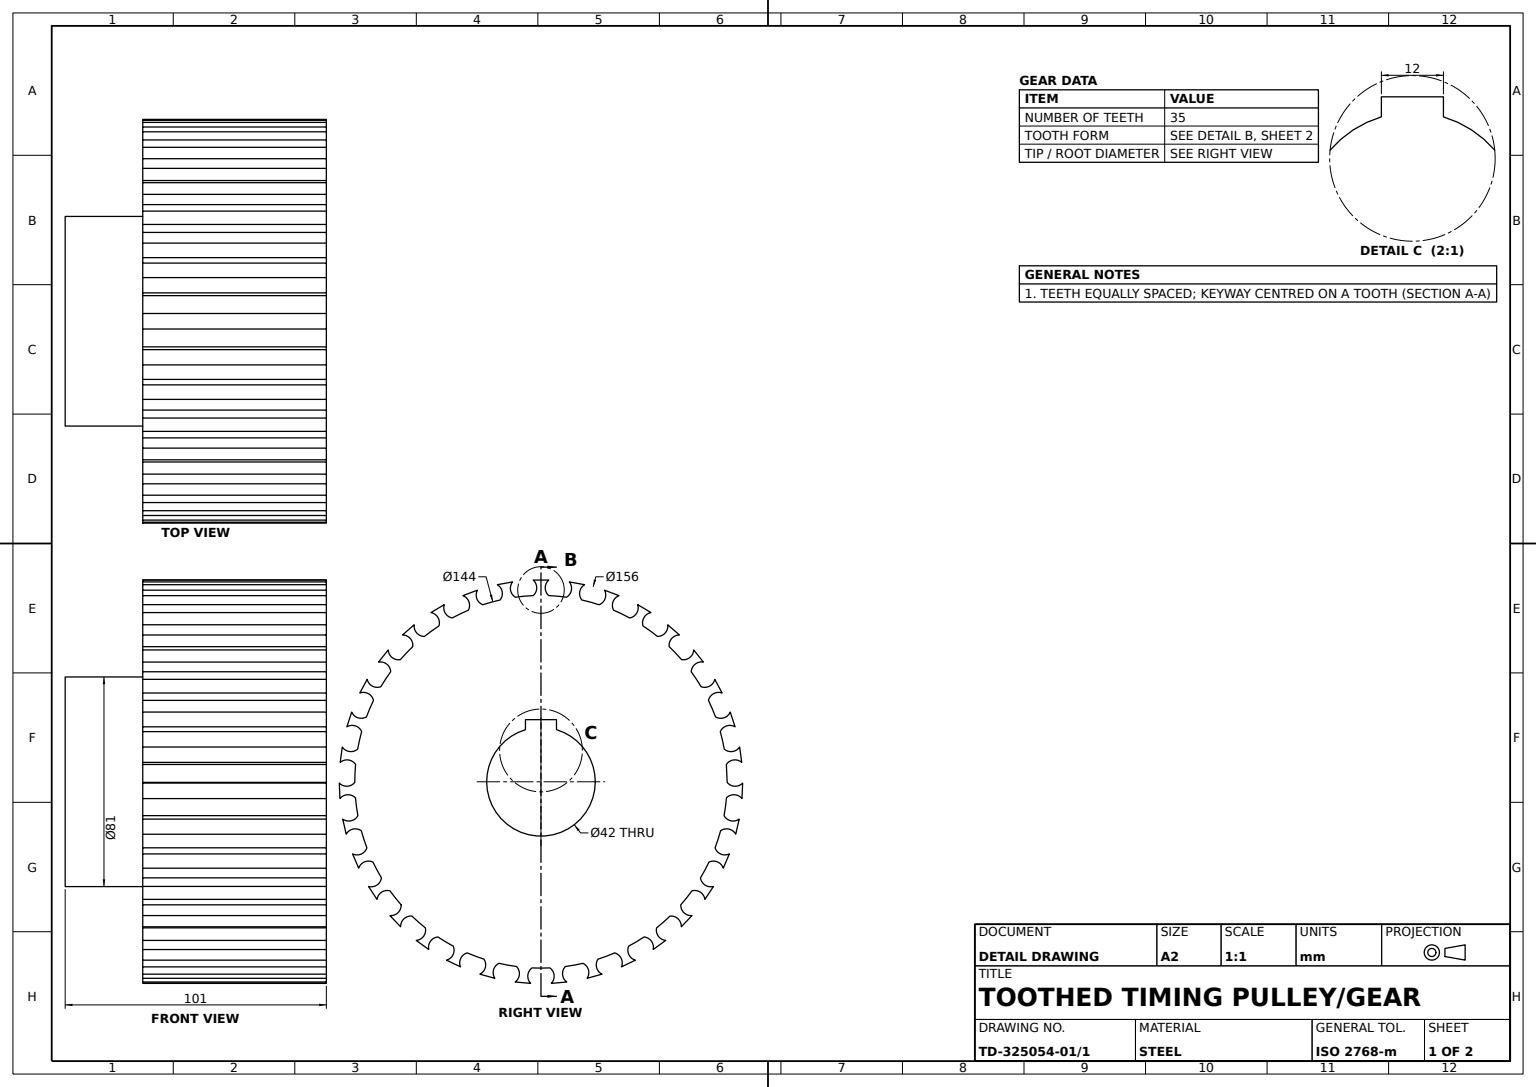
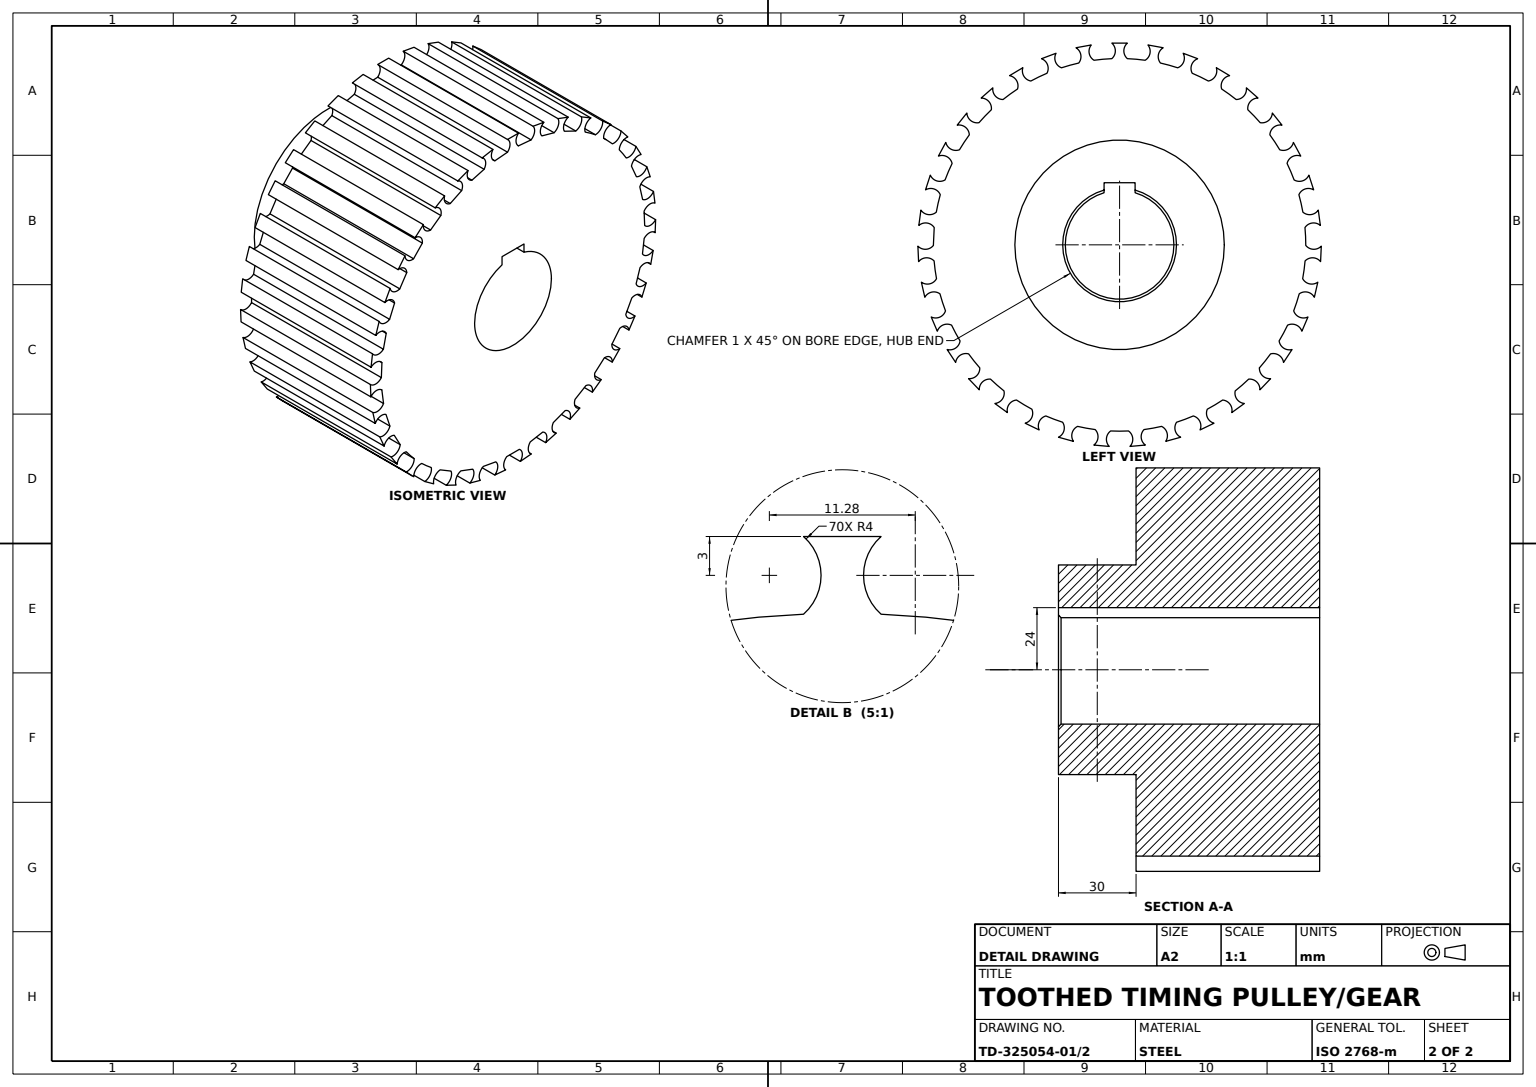
SolidWorks part; units mm, degrees
material "Plain Carbon Steel"
ref_plane "Front Plane" through (0, 0, 0) normal (0, 0, 1) x (1, 0, 0)
ref_plane "Top Plane" through (0, 0, 0) normal (0, 1, 0) x (1, 0, 0)
ref_plane "Right Plane" through (0, 0, 0) normal (1, 0, 0) x (0, 0, -1)
sketch "Gear Tooth Profile Sketch" plane through (0, 0, 0) normal (0, 0, 1) x (1, 0, 0)
  line L0 (0, 0) -> (0, 72) construction
  line L3 (0, 72) -> (0, 83.2045)
  line L4 (-2.9993, 80.7614) -> (-2.9993, 80.6935) construction
  arc A0 (2.9993, 77.9423) -> (-2.9993, 77.9423) centre (0, 0) ccw
  arc A1 (-2.9993, 71.9375) -> (-9.8938, 71.317) centre (0, 0) ccw
  circle A2 centre (0, 0) radius 64.8
  arc A3 (2.9993, 71.9375) -> (2.9993, 77.9423) centre (5.6424, 74.9399) cw
  arc A4 (-2.9993, 71.9375) -> (-2.9993, 77.9423) centre (-5.6424, 74.9399) ccw
  arc A5 (9.8938, 71.317) -> (10.966, 77.2253) centre (7.8293, 74.7431) ccw
  arc A6 (15.7961, 70.2459) -> (16.8683, 76.1542) centre (18.9327, 72.7281) cw
  arc A7 (22.4689, 68.4043) -> (24.5789, 74.0262) centre (21.0494, 72.1439) ccw
  arc A8 (28.0851, 66.2965) -> (30.1951, 71.9184) centre (31.6146, 68.1788) cw
  arc A9 (34.3219, 63.293) -> (37.4018, 68.4478) centre (33.5929, 67.226) ccw
  arc A10 (39.4715, 60.2163) -> (42.5513, 65.3711) centre (43.2803, 61.4381) cw
  arc A11 (45.0717, 56.1475) -> (49.0225, 60.6695) centre (45.0568, 60.1474) ccw
  arc A12 (49.5892, 52.2007) -> (53.54, 56.7227) centre (53.555, 52.7228) cw
  arc A13 (54.3729, 47.1973) -> (59.0677, 50.9412) centre (55.0724, 51.1356) ccw
  arc A14 (58.1131, 42.5073) -> (62.8078, 46.2513) centre (62.1083, 42.3129) cw
  arc A15 (61.9265, 36.7301) -> (67.2144, 39.5756) centre (63.318, 40.4803) ccw
  arc A16 (64.7691, 31.4477) -> (70.0569, 34.2932) centre (68.6655, 30.543) cw
  arc A17 (67.4898, 25.0825) -> (73.2007, 26.938) centre (69.5285, 28.5239) ccw
  arc A18 (69.3435, 19.3774) -> (75.0544, 21.2329) centre (73.0157, 17.7915) cw
  arc A19 (70.8838, 12.6286) -> (76.8343, 13.4347) centre (73.5043, 15.6507) ccw
  arc A20 (71.6891, 6.6842) -> (77.6395, 7.4902) centre (75.0191, 4.4681) cw
  arc A21 (71.9996, -0.2311) -> (77.9984, -0.5005) centre (75.1176, 2.2745) ccw
  arc A22 (71.7305, -6.2238) -> (77.7293, -6.4932) centre (74.6113, -8.9989) cw
  arc A23 (70.8013, -13.0835) -> (76.6556, -14.4196) centre (74.3166, -11.1748) ccw
  arc A24 (69.4665, -18.9317) -> (75.3207, -20.2679) centre (71.8055, -22.1766) cw
  arc A25 (67.3273, -25.5153) -> (72.8489, -27.8753) centre (71.1269, -24.2649) ccw
  arc A26 (64.9697, -31.0312) -> (70.4913, -33.3913) centre (66.6917, -34.6416) cw
  arc A27 (61.6894, -37.127) -> (66.7009, -40.435) centre (65.6512, -36.5752) ccw
  arc A28 (58.3848, -42.1333) -> (63.3962, -45.4414) centre (59.4345, -45.9931) cw
  arc A29 (54.0688, -47.5454) -> (58.409, -51.6951) centre (58.0654, -47.7099) ccw
  arc A30 (49.9233, -51.8812) -> (54.2636, -56.0309) centre (50.2669, -55.8664) cw
  arc A31 (44.7103, -56.4357) -> (48.2399, -61.2937) centre (48.6133, -57.3112) ccw
  arc A32 (39.8573, -59.9616) -> (43.3868, -64.8196) centre (39.4838, -63.9442) cw
  arc A33 (33.9148, -63.5121) -> (36.5202, -68.9222) centre (37.5988, -65.0704) ccw
  arc A34 (28.5102, -66.1148) -> (31.1156, -71.525) centre (27.4316, -69.9667) cw
  arc A35 (22.0293, -68.5471) -> (23.6268, -74.3356) centre (25.3758, -70.7382) ccw
  arc A36 (16.2468, -70.143) -> (17.8443, -75.9314) centre (14.4977, -73.7404) cw
  arc A37 (9.4357, -71.379) -> (9.974, -77.3597) centre (12.3372, -74.1324) ccw
  arc A38 (3.4612, -71.9168) -> (3.9994, -77.8974) centre (1.0979, -75.144) cw
  arc A39 (-3.4612, -71.9168) -> (-3.9994, -77.8974) centre (-1.0979, -75.144) ccw
  arc A40 (-9.4357, -71.379) -> (-9.974, -77.3597) centre (-12.3372, -74.1324) cw
  arc A41 (-16.2468, -70.143) -> (-17.8443, -75.9314) centre (-14.4977, -73.7404) ccw
  arc A42 (-22.0293, -68.5471) -> (-23.6268, -74.3356) centre (-25.3758, -70.7382) cw
  arc A43 (-28.5102, -66.1148) -> (-31.1156, -71.525) centre (-27.4316, -69.9667) ccw
  arc A44 (-33.9148, -63.5121) -> (-36.5202, -68.9222) centre (-37.5988, -65.0704) cw
  arc A45 (-39.8573, -59.9616) -> (-43.3868, -64.8196) centre (-39.4838, -63.9442) ccw
  arc A46 (-44.7103, -56.4357) -> (-48.2399, -61.2937) centre (-48.6133, -57.3112) cw
  arc A47 (-49.9233, -51.8812) -> (-54.2636, -56.0309) centre (-50.2669, -55.8664) ccw
  arc A48 (-54.0688, -47.5454) -> (-58.409, -51.6951) centre (-58.0654, -47.7099) cw
  arc A49 (-58.3848, -42.1333) -> (-63.3962, -45.4414) centre (-59.4345, -45.9931) ccw
  arc A50 (-61.6894, -37.127) -> (-66.7009, -40.435) centre (-65.6512, -36.5752) cw
  arc A51 (-64.9697, -31.0312) -> (-70.4913, -33.3913) centre (-66.6917, -34.6416) ccw
  arc A52 (-67.3273, -25.5153) -> (-72.8489, -27.8753) centre (-71.1269, -24.2649) cw
  arc A53 (-69.4665, -18.9317) -> (-75.3207, -20.2679) centre (-71.8055, -22.1766) ccw
  arc A54 (-70.8013, -13.0835) -> (-76.6556, -14.4196) centre (-74.3166, -11.1748) cw
  arc A55 (-71.7305, -6.2238) -> (-77.7293, -6.4932) centre (-74.6113, -8.9989) ccw
  arc A56 (-71.9996, -0.2311) -> (-77.9984, -0.5005) centre (-75.1176, 2.2745) cw
  arc A57 (-71.6891, 6.6842) -> (-77.6395, 7.4902) centre (-75.0191, 4.4681) ccw
  arc A58 (-70.8838, 12.6286) -> (-76.8343, 13.4347) centre (-73.5043, 15.6507) cw
  arc A59 (-69.3435, 19.3774) -> (-75.0544, 21.2329) centre (-73.0157, 17.7915) ccw
  arc A60 (-67.4898, 25.0825) -> (-73.2007, 26.938) centre (-69.5285, 28.5239) cw
  arc A61 (-64.7691, 31.4477) -> (-70.0569, 34.2932) centre (-68.6655, 30.543) ccw
  arc A62 (-61.9265, 36.7301) -> (-67.2144, 39.5756) centre (-63.318, 40.4803) cw
  arc A63 (-58.1131, 42.5073) -> (-62.8078, 46.2513) centre (-62.1083, 42.3129) ccw
  arc A64 (-54.3729, 47.1973) -> (-59.0677, 50.9412) centre (-55.0724, 51.1356) cw
  arc A65 (-49.5892, 52.2007) -> (-53.54, 56.7227) centre (-53.555, 52.7228) ccw
  arc A66 (-45.0717, 56.1475) -> (-49.0225, 60.6695) centre (-45.0568, 60.1474) cw
  arc A67 (-39.4715, 60.2163) -> (-42.5513, 65.3711) centre (-43.2803, 61.4381) ccw
  arc A68 (-34.3219, 63.293) -> (-37.4018, 68.4478) centre (-33.5929, 67.226) cw
  arc A69 (-28.0851, 66.2965) -> (-30.1951, 71.9184) centre (-31.6146, 68.1788) ccw
  arc A70 (-22.4689, 68.4043) -> (-24.5789, 74.0262) centre (-21.0494, 72.1439) cw
  arc A71 (-15.7961, 70.2459) -> (-16.8683, 76.1542) centre (-18.9327, 72.7281) ccw
  arc A72 (-9.8938, 71.317) -> (-10.966, 77.2253) centre (-7.8293, 74.7431) cw
  arc A73 (16.8683, 76.1542) -> (10.966, 77.2253) centre (0, 0) ccw
  arc A74 (30.1951, 71.9184) -> (24.5789, 74.0262) centre (0, 0) ccw
  arc A75 (42.5513, 65.3711) -> (37.4018, 68.4478) centre (0, 0) ccw
  arc A76 (53.54, 56.7227) -> (49.0225, 60.6695) centre (0, 0) ccw
  arc A77 (62.8078, 46.2513) -> (59.0677, 50.9412) centre (0, 0) ccw
  arc A78 (70.0569, 34.2932) -> (67.2144, 39.5756) centre (0, 0) ccw
  arc A79 (75.0544, 21.2329) -> (73.2007, 26.938) centre (0, 0) ccw
  arc A80 (77.6395, 7.4902) -> (76.8343, 13.4347) centre (0, 0) ccw
  arc A81 (77.7293, -6.4932) -> (77.9984, -0.5005) centre (0, 0) ccw
  arc A82 (75.3207, -20.2679) -> (76.6556, -14.4196) centre (0, 0) ccw
  arc A83 (70.4913, -33.3913) -> (72.8489, -27.8753) centre (0, 0) ccw
  arc A84 (63.3962, -45.4414) -> (66.7009, -40.435) centre (0, 0) ccw
  arc A85 (54.2636, -56.0309) -> (58.409, -51.6951) centre (0, 0) ccw
  arc A86 (43.3868, -64.8196) -> (48.2399, -61.2937) centre (0, 0) ccw
  arc A87 (31.1156, -71.525) -> (36.5202, -68.9222) centre (0, 0) ccw
  arc A88 (17.8443, -75.9314) -> (23.6268, -74.3356) centre (0, 0) ccw
  arc A89 (3.9994, -77.8974) -> (9.974, -77.3597) centre (0, 0) ccw
  arc A90 (-9.974, -77.3597) -> (-3.9994, -77.8974) centre (0, 0) ccw
  arc A91 (-23.6268, -74.3356) -> (-17.8443, -75.9314) centre (0, 0) ccw
  arc A92 (-36.5202, -68.9222) -> (-31.1156, -71.525) centre (0, 0) ccw
  arc A93 (-48.2399, -61.2937) -> (-43.3868, -64.8196) centre (0, 0) ccw
  arc A94 (-58.409, -51.6951) -> (-54.2636, -56.0309) centre (0, 0) ccw
  arc A95 (-66.7009, -40.435) -> (-63.3962, -45.4414) centre (0, 0) ccw
  arc A96 (-72.8489, -27.8753) -> (-70.4913, -33.3913) centre (0, 0) ccw
  arc A97 (-76.6556, -14.4196) -> (-75.3207, -20.2679) centre (0, 0) ccw
  arc A98 (-77.9984, -0.5005) -> (-77.7293, -6.4932) centre (0, 0) ccw
  arc A99 (-76.8343, 13.4347) -> (-77.6395, 7.4902) centre (0, 0) ccw
  arc A100 (-73.2007, 26.938) -> (-75.0544, 21.2329) centre (0, 0) ccw
  arc A101 (-67.2144, 39.5756) -> (-70.0569, 34.2932) centre (0, 0) ccw
  arc A102 (-59.0677, 50.9412) -> (-62.8078, 46.2513) centre (0, 0) ccw
  arc A103 (-49.0225, 60.6695) -> (-53.54, 56.7227) centre (0, 0) ccw
  arc A104 (-37.4018, 68.4478) -> (-42.5513, 65.3711) centre (0, 0) ccw
  arc A105 (-24.5789, 74.0262) -> (-30.1951, 71.9184) centre (0, 0) ccw
  arc A106 (-10.966, 77.2253) -> (-16.8683, 76.1542) centre (0, 0) ccw
  arc A107 (9.8938, 71.317) -> (2.9993, 71.9375) centre (0, 0) ccw
  arc A108 (22.4689, 68.4043) -> (15.7961, 70.2459) centre (0, 0) ccw
  arc A109 (34.3219, 63.293) -> (28.0851, 66.2965) centre (0, 0) ccw
  arc A110 (45.0717, 56.1475) -> (39.4715, 60.2163) centre (0, 0) ccw
  arc A111 (54.3729, 47.1973) -> (49.5892, 52.2007) centre (0, 0) ccw
  arc A112 (61.9265, 36.7301) -> (58.1131, 42.5073) centre (0, 0) ccw
  arc A113 (67.4898, 25.0825) -> (64.7691, 31.4477) centre (0, 0) ccw
  arc A114 (70.8838, 12.6286) -> (69.3435, 19.3774) centre (0, 0) ccw
  arc A115 (71.9996, -0.2311) -> (71.6891, 6.6842) centre (0, 0) ccw
  arc A116 (70.8013, -13.0835) -> (71.7305, -6.2238) centre (0, 0) ccw
  arc A117 (67.3273, -25.5153) -> (69.4665, -18.9317) centre (0, 0) ccw
  arc A118 (61.6894, -37.127) -> (64.9697, -31.0312) centre (0, 0) ccw
  arc A119 (54.0688, -47.5454) -> (58.3848, -42.1333) centre (0, 0) ccw
  arc A120 (44.7103, -56.4357) -> (49.9233, -51.8812) centre (0, 0) ccw
  arc A121 (33.9148, -63.5121) -> (39.8573, -59.9616) centre (0, 0) ccw
  arc A122 (22.0293, -68.5471) -> (28.5102, -66.1148) centre (0, 0) ccw
  arc A123 (9.4357, -71.379) -> (16.2468, -70.143) centre (0, 0) ccw
  arc A124 (-3.4612, -71.9168) -> (3.4612, -71.9168) centre (0, 0) ccw
  arc A125 (-16.2468, -70.143) -> (-9.4357, -71.379) centre (0, 0) ccw
  arc A126 (-28.5102, -66.1148) -> (-22.0293, -68.5471) centre (0, 0) ccw
  arc A127 (-39.8573, -59.9616) -> (-33.9148, -63.5121) centre (0, 0) ccw
  arc A128 (-49.9233, -51.8812) -> (-44.7103, -56.4357) centre (0, 0) ccw
  arc A129 (-58.3848, -42.1333) -> (-54.0688, -47.5454) centre (0, 0) ccw
  arc A130 (-64.9697, -31.0312) -> (-61.6894, -37.127) centre (0, 0) ccw
  arc A131 (-69.4665, -18.9317) -> (-67.3273, -25.5153) centre (0, 0) ccw
  arc A132 (-71.7305, -6.2238) -> (-70.8013, -13.0835) centre (0, 0) ccw
  arc A133 (-71.6891, 6.6842) -> (-71.9996, -0.2311) centre (0, 0) ccw
  arc A134 (-69.3435, 19.3774) -> (-70.8838, 12.6286) centre (0, 0) ccw
  arc A135 (-64.7691, 31.4477) -> (-67.4898, 25.0825) centre (0, 0) ccw
  arc A136 (-58.1131, 42.5073) -> (-61.9265, 36.7301) centre (0, 0) ccw
  arc A137 (-49.5892, 52.2007) -> (-54.3729, 47.1973) centre (0, 0) ccw
  arc A138 (-39.4715, 60.2163) -> (-45.0717, 56.1475) centre (0, 0) ccw
  arc A139 (-28.0851, 66.2965) -> (-34.3219, 63.293) centre (0, 0) ccw
  arc A140 (-15.7961, 70.2459) -> (-22.4689, 68.4043) centre (0, 0) ccw
  dimension "D1" = 156
  dimension "D2" = 144
  dimension "D3" = 129.6
  dimension "D4" = 4
  dimension "D5" = 4
  dimension "D6" = 35
  dimension "D7" = 5.6424
  dimension "D8" = 74.9399
  dimension "D9" = 83.2045
  dimension "D10" = 2.9993
extrude "Gear Body 35T" add sketch "Gear Tooth Profile Sketch" along normal blind 71 contours A76 A11 A110 A10 A75 A9 A109 A8 A74 A7 A108 A6 A73 A5 A107 A3 A0 A4 A1 A72 A106 A71 A140 A70 A105 A69 A139 A68 A104 A67 A138 A66 A103 A65 A137 A64 A102 A63 A136 A62 A101 A61 A135 A60 A100 A59 A134 A58 A99 A57 A133 A56 A98 A55 A132 A54 A97 A53 A131 A52 A96 A51 A130 A50 A95 A49 A129 A48 A94 A47 A128 A46 A93 A45 A127 A44 A92 A43 A126 A42 A91 A41 A125 A40 A90 A39 A124 A38 A89 A37 A123 A36 A88 A35 A122 A34 A87 A33 A121 A32 A86 A31 A120 A30 A85 A29 A119 A28 A84 A27 A118 A26 A83 A25 A117 A24 A82 A23 A116 A22 A81 A21 A115 A20 A80 A19 A114 A18 A79 A17 A113 A16 A78 A15 A112 A14 A77 A13 A111 A12
sketch "Hub Sketch" plane through (0, 0, 71) normal (0, 0, 1) x (1, 0, 0)
  circle A0 centre (0, 0) radius 40.5
  dimension "D1" = 81
extrude "Hub Ø81" add sketch "Hub Sketch" along normal blind 30
sketch "Bore Keyway Sketch" plane through (0, 0, 101) normal (0, 0, 1) x (1, 0, 0)
  line L1 (-6, 24) -> (6, 24)
  line L2 (-6, 24) -> (-6, 20.1246)
  line L4 (6, 24) -> (6, 20.1246)
  arc A0 (-6, 20.1246) -> (6, 20.1246) centre (0, 0) ccw
  circle A1 centre (0, 0) radius 40.5 construction
  point P3 (0, 21)
  dimension "D1" = 42
  dimension "D2" = 6
  dimension "D3" = 24
extrude "Bore Ø42 with Keyway" cut sketch "Bore Keyway Sketch" against normal through all
chamfer "Edge Chamfer 1x45" distance 1 angle 45 1 edges at (0, -21, 101)
